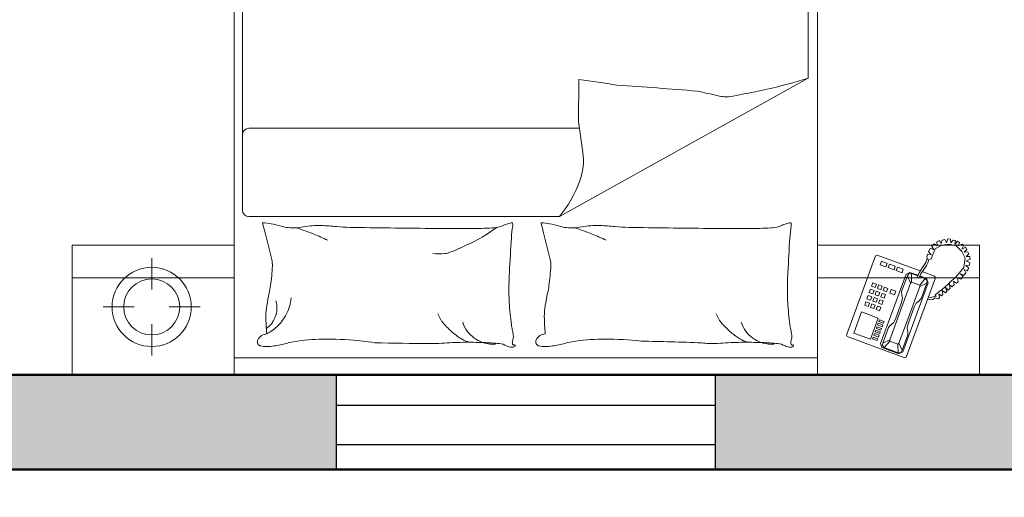
# Model space of a CAD drawing. Units: inches. Extents: x -7 to 1228, y -146 to 1091.
# Tile 17 of 88: x 420 to 513, y 57 to 103. Entities that reach past the tile are written whole.
import ezdxf

# ---------------------------------------------------------------- set-up
doc = ezdxf.new("R2010")
doc.units = ezdxf.units.IN
for name, color, linetype, lineweight in [('A-ANNO-DIMS', 2, 'Continuous', 18), ('A-FURN', 8, 'Continuous', 18), ('A-GLAZ', 175, 'Continuous', 25), ('A-WALL', 7, 'Continuous', 50), ('A-WALL-PATT', 251, 'Continuous', 13)]:
    doc.layers.add(name, color=color, linetype=linetype, lineweight=lineweight)
doc.styles.add('DIM_FONT', font='SIMPLEX.shx', dxfattribs={"width": 0.8})
doc.styles.get("Standard").update_dxf_attribs({"font": 'arial.ttf'})
doc.dimstyles.new('ISO-25', dxfattribs={"dimtxt": 7, "dimasz": 4, "dimexe": 1.25, "dimexo": 0.625, "dimtad": 1, "dimdec": 1, "dimlunit": 3, "dimtxsty": 'Standard', "dimcen": 2.5, "dimadec": 0, "dimazin": 0, "dimtfac": 1, "dimtdec": 1, "dimtmove": 1, "dimatfit": 3, "dimfxl": 1, "dimarcsym": 0})

# ---------------------------------------------------------------- blocks, each defined once
blk = doc.blocks.new('A$C4F634EDD')
for p, q in [((0, 2.6295), (0, 2.2295)), ((0.5, 2.6295), (0, 2.6295)), ((0.5, 2.6295), (2.3, 2.6295)), ((0.5, 0.5295), (0.5, 2.6295)), ((0.5, 2.2295), (0.5, 2.6295)), ((2.3, 2.6295), (2.3, 0.5295)), ((2.3, 2.6295), (2.8, 2.6295)), ((2.3, 2.2295), (2.3, 2.6295)), ((2.8, 2.6295), (2.8, 2.2295)), ((0.2457, 2.5697), (0.2457, 2.4733)), ((0.5, 2.5771), (2.3, 2.5771)), ((2.392, 2.5115), (2.5692, 2.5765)), ((2.4985, 2.5445), (2.5516, 2.564)), ((2.5062, 2.5454), (2.5487, 2.561)), ((2.5483, 2.5347), (2.5487, 2.561)), ((2.5487, 2.561), (2.5571, 2.56)), ((2.5615, 2.5536), (2.5514, 2.5318)), ((2.5516, 2.564), (2.5637, 2.5584)), ((2.5571, 2.56), (2.5615, 2.5536)), ((2.5615, 2.5536), (2.5791, 2.5058)), ((2.5637, 2.5584), (2.6418, 2.3458)), ((2.5692, 2.5765), (2.574, 2.5743)), ((2.574, 2.5743), (2.6638, 2.3298)), ((2.4842, 2.5232), (2.47, 2.518)), ((2.4862, 2.5179), (2.4842, 2.5232)), ((2.4946, 2.5331), (2.4985, 2.5445)), ((2.5734, 2.3187), (2.4946, 2.5331)), ((2.5062, 2.5454), (2.5004, 2.5392)), ((2.5004, 2.5392), (2.5013, 2.5315)), ((2.5013, 2.5315), (2.5188, 2.4836)), ((2.5013, 2.5315), (2.5231, 2.5214)), ((2.5235, 2.5256), (2.5062, 2.5454)), ((2.5231, 2.5214), (2.5235, 2.5256)), ((2.5483, 2.5347), (2.5235, 2.5256)), ((2.5514, 2.5318), (2.5483, 2.5347)), ((2.5807, 2.4521), (2.5514, 2.5318)), ((2.3898, 2.5066), (2.392, 2.5115)), ((2.4795, 2.2621), (2.3898, 2.5066)), ((2.412, 2.5007), (2.4634, 2.5196)), ((2.4361, 2.4352), (2.412, 2.5007)), ((2.4634, 2.5196), (2.4875, 2.454)), ((2.47, 2.518), (2.472, 2.5127)), ((2.472, 2.5127), (2.4862, 2.5179)), ((2.4881, 2.5126), (2.4739, 2.5074)), ((2.4739, 2.5074), (2.4759, 2.502)), ((2.4759, 2.502), (2.4901, 2.5073)), ((2.492, 2.5019), (2.4778, 2.4967)), ((2.4778, 2.4967), (2.4798, 2.4914)), ((2.4798, 2.4914), (2.494, 2.4966)), ((2.4901, 2.5073), (2.4881, 2.5126)), ((2.494, 2.4966), (2.492, 2.5019)), ((2.5523, 2.4417), (2.5231, 2.5214)), ((2.5788, 2.4956), (2.5767, 2.4848)), ((2.5791, 2.5058), (2.5788, 2.4956)), ((2.4959, 2.4913), (2.4817, 2.4861)), ((2.4817, 2.4861), (2.4837, 2.4808)), ((2.4837, 2.4808), (2.4979, 2.486)), ((2.4998, 2.4807), (2.4856, 2.4755)), ((2.4856, 2.4755), (2.4876, 2.4702)), ((2.4876, 2.4702), (2.5018, 2.4754)), ((2.5037, 2.47), (2.4895, 2.4648)), ((2.4895, 2.4648), (2.4915, 2.4595)), ((2.4915, 2.4595), (2.5057, 2.4647)), ((2.4979, 2.486), (2.4959, 2.4913)), ((2.5018, 2.4754), (2.4998, 2.4807)), ((2.5057, 2.4647), (2.5037, 2.47)), ((2.5188, 2.4836), (2.5256, 2.4761)), ((2.5256, 2.4761), (2.5342, 2.4692)), ((2.5342, 2.4692), (2.5405, 2.4574)), ((2.5767, 2.4848), (2.5795, 2.4717)), ((2.5795, 2.4717), (2.586, 2.454)), ((2.4875, 2.454), (2.4361, 2.4352)), ((2.4811, 2.4276), (2.4917, 2.4315)), ((2.4917, 2.4315), (2.4956, 2.4208)), ((2.5405, 2.4574), (2.547, 2.4397)), ((2.5594, 2.4061), (2.547, 2.4397)), ((2.5523, 2.4417), (2.5875, 2.346)), ((2.5807, 2.4521), (2.6158, 2.3564)), ((2.5984, 2.4204), (2.586, 2.454)), ((0.0957, 2.4197), (0.192, 2.4197)), ((0.2994, 2.4197), (0.3957, 2.4197)), ((2.4457, 2.4146), (2.4563, 2.4185)), ((2.4496, 2.4039), (2.4457, 2.4146)), ((2.4602, 2.4078), (2.4496, 2.4039)), ((2.4563, 2.4185), (2.4602, 2.4078)), ((2.4634, 2.4211), (2.474, 2.425)), ((2.4673, 2.4104), (2.4634, 2.4211)), ((2.4779, 2.4143), (2.4673, 2.4104)), ((2.4706, 2.4016), (2.4812, 2.4055)), ((2.4745, 2.3909), (2.4706, 2.4016)), ((2.474, 2.425), (2.4779, 2.4143)), ((2.485, 2.4169), (2.4811, 2.4276)), ((2.4812, 2.4055), (2.4851, 2.3949)), ((2.4956, 2.4208), (2.485, 2.4169)), ((2.4883, 2.4081), (2.4989, 2.412)), ((2.4922, 2.3975), (2.4883, 2.4081)), ((2.5028, 2.4014), (2.4922, 2.3975)), ((2.4989, 2.412), (2.5028, 2.4014)), ((2.5622, 2.393), (2.5594, 2.4061)), ((2.6047, 2.4086), (2.5984, 2.4204)), ((2.6133, 2.4017), (2.6047, 2.4086)), ((2.6201, 2.3941), (2.6133, 2.4017)), ((2.4528, 2.3951), (2.4635, 2.399)), ((2.4567, 2.3844), (2.4528, 2.3951)), ((2.4674, 2.3883), (2.4567, 2.3844)), ((2.46, 2.3756), (2.4706, 2.3795)), ((2.4639, 2.365), (2.46, 2.3756)), ((2.4635, 2.399), (2.4674, 2.3883)), ((2.4706, 2.3795), (2.4745, 2.3689)), ((2.4851, 2.3949), (2.4745, 2.3909)), ((2.4777, 2.3821), (2.4883, 2.386)), ((2.4816, 2.3715), (2.4777, 2.3821)), ((2.4922, 2.3754), (2.4816, 2.3715)), ((2.4883, 2.386), (2.4922, 2.3754)), ((2.4954, 2.3886), (2.5061, 2.3925)), ((2.4993, 2.378), (2.4954, 2.3886)), ((2.51, 2.3819), (2.4993, 2.378)), ((2.5026, 2.3691), (2.5132, 2.373)), ((2.5061, 2.3925), (2.51, 2.3819)), ((2.5132, 2.373), (2.5171, 2.3624)), ((2.5238, 2.3769), (2.538, 2.3821)), ((2.5277, 2.3663), (2.5238, 2.3769)), ((2.5419, 2.3715), (2.5277, 2.3663)), ((2.538, 2.3821), (2.5419, 2.3715)), ((2.5598, 2.372), (2.5601, 2.3822)), ((2.5774, 2.3242), (2.5598, 2.372)), ((2.5601, 2.3822), (2.5622, 2.393)), ((2.6376, 2.3463), (2.6201, 2.3941)), ((2.6499, 2.3979), (2.6397, 2.3953)), ((2.6417, 2.39), (2.6488, 2.391)), ((2.6488, 2.391), (2.6538, 2.3895)), ((2.6551, 2.397), (2.6499, 2.3979)), ((2.6538, 2.3895), (2.6596, 2.388)), ((2.6627, 2.392), (2.6551, 2.397)), ((2.6596, 2.388), (2.6626, 2.3867)), ((2.6626, 2.3867), (2.6662, 2.388)), ((2.6692, 2.394), (2.6627, 2.392)), ((2.6662, 2.388), (2.6632, 2.3828)), ((2.6632, 2.3828), (2.6736, 2.3744)), ((2.6736, 2.3944), (2.6692, 2.394)), ((2.6765, 2.391), (2.6736, 2.3944)), ((2.6736, 2.3744), (2.6922, 2.3593)), ((2.6742, 2.3795), (2.6765, 2.391)), ((2.6824, 2.3858), (2.6742, 2.3795)), ((2.6873, 2.3815), (2.6824, 2.3858)), ((2.6853, 2.369), (2.6873, 2.3815)), ((2.6946, 2.376), (2.6853, 2.369)), ((2.6995, 2.3713), (2.6946, 2.376)), ((2.695, 2.3603), (2.6995, 2.3713)), ((0.2457, 2.366), (0.2457, 2.2697)), ((2.4745, 2.3689), (2.4639, 2.365)), ((2.4672, 2.3561), (2.4778, 2.36)), ((2.4711, 2.3455), (2.4672, 2.3561)), ((2.4817, 2.3494), (2.4711, 2.3455)), ((2.4778, 2.36), (2.4817, 2.3494)), ((2.4849, 2.3626), (2.4955, 2.3665)), ((2.4888, 2.352), (2.4849, 2.3626)), ((2.4994, 2.3559), (2.4888, 2.352)), ((2.4955, 2.3665), (2.4994, 2.3559)), ((2.5065, 2.3585), (2.5026, 2.3691)), ((2.5171, 2.3624), (2.5065, 2.3585)), ((2.5774, 2.3242), (2.5875, 2.346)), ((2.5875, 2.346), (2.5905, 2.3431)), ((2.5905, 2.3431), (2.5901, 2.3168)), ((2.6154, 2.3522), (2.5905, 2.3431)), ((2.6158, 2.3564), (2.6154, 2.3522)), ((2.6154, 2.3522), (2.6327, 2.3324)), ((2.6376, 2.3463), (2.6158, 2.3564)), ((2.6418, 2.3458), (2.6369, 2.332)), ((2.6385, 2.3386), (2.6376, 2.3463)), ((2.6922, 2.3593), (2.7051, 2.3473)), ((2.7031, 2.3682), (2.695, 2.3603)), ((2.7096, 2.3616), (2.7031, 2.3682)), ((2.7051, 2.3473), (2.7079, 2.3475)), ((2.7062, 2.351), (2.7096, 2.3616)), ((2.7147, 2.3578), (2.7062, 2.351)), ((2.7079, 2.3475), (2.7079, 2.3443)), ((2.7079, 2.3443), (2.727, 2.3277)), ((2.7214, 2.3517), (2.7147, 2.3578)), ((2.7196, 2.34), (2.7214, 2.3517)), ((2.7286, 2.3466), (2.7196, 2.34)), ((2.7346, 2.3423), (2.7286, 2.3466)), ((2.732, 2.3295), (2.7346, 2.3423)), ((0, 2.3301), (0.5, 2.3301)), ((2.8, 2.3301), (2.3, 2.3301)), ((2.561, 2.3141), (2.5433, 2.3076)), ((2.5649, 2.3035), (2.561, 2.3141)), ((2.5855, 2.3131), (2.5734, 2.3187)), ((2.5818, 2.3178), (2.5774, 2.3242)), ((2.5901, 2.3168), (2.5818, 2.3178)), ((2.6104, 2.3222), (2.5855, 2.3131)), ((2.5901, 2.3168), (2.6097, 2.324)), ((2.613, 2.3312), (2.6077, 2.3293)), ((2.6077, 2.3293), (2.6135, 2.3141)), ((2.6192, 2.3174), (2.613, 2.3312)), ((2.6135, 2.3141), (2.6244, 2.2977)), ((2.6153, 2.3261), (2.6327, 2.3324)), ((2.6369, 2.332), (2.6161, 2.3243)), ((2.626, 2.3069), (2.6192, 2.3174)), ((2.6616, 2.3249), (2.6234, 2.3109)), ((2.6327, 2.3324), (2.6385, 2.3386)), ((2.6638, 2.3298), (2.6616, 2.3249)), ((2.727, 2.3277), (2.7512, 2.2983)), ((2.7423, 2.3345), (2.732, 2.3295)), ((2.7406, 2.3172), (2.7495, 2.325)), ((2.7519, 2.3218), (2.7406, 2.3172)), ((2.7495, 2.325), (2.7423, 2.3345)), ((2.7575, 2.3144), (2.7519, 2.3218)), ((2.7526, 2.3045), (2.7575, 2.3144)), ((2.6172, 2.3086), (2.4844, 2.2599)), ((2.5114, 2.2959), (2.4936, 2.2894)), ((2.4936, 2.2894), (2.4976, 2.2788)), ((2.4976, 2.2788), (2.5153, 2.2853)), ((2.5153, 2.2853), (2.5114, 2.2959)), ((2.5362, 2.305), (2.5185, 2.2985)), ((2.5185, 2.2985), (2.5224, 2.2879)), ((2.5224, 2.2879), (2.5401, 2.2944)), ((2.5401, 2.2944), (2.5362, 2.305)), ((2.5433, 2.3076), (2.5472, 2.297)), ((2.5472, 2.297), (2.5649, 2.3035)), ((2.6244, 2.2977), (2.6349, 2.2825)), ((2.6365, 2.2916), (2.626, 2.3069)), ((2.6349, 2.2825), (2.638, 2.273)), ((2.6407, 2.2834), (2.6365, 2.2916)), ((2.6438, 2.2739), (2.6407, 2.2834)), ((2.7512, 2.2983), (2.756, 2.2695)), ((2.7622, 2.308), (2.7526, 2.3045)), ((2.7574, 2.2924), (2.7673, 2.2997)), ((2.7687, 2.2905), (2.7574, 2.2924)), ((2.7587, 2.279), (2.7699, 2.2828)), ((2.7708, 2.2725), (2.7587, 2.279)), ((2.7673, 2.2997), (2.7622, 2.308)), ((2.7699, 2.2828), (2.7687, 2.2905)), ((0.5953, 2.1912), (0.616, 2.2738)), ((1.4546, 2.1912), (1.4752, 2.2738)), ((2.4844, 2.2599), (2.4795, 2.2621)), ((2.6399, 2.2712), (2.6374, 2.2659)), ((2.6374, 2.2659), (2.6398, 2.257)), ((2.638, 2.273), (2.6399, 2.2712)), ((2.6398, 2.257), (2.6509, 2.259)), ((2.6509, 2.259), (2.6431, 2.2492)), ((2.6431, 2.2492), (2.6473, 2.2398)), ((2.6519, 2.2716), (2.6438, 2.2739)), ((2.6535, 2.2628), (2.6519, 2.2716)), ((2.6636, 2.2409), (2.6535, 2.2628)), ((2.7459, 2.2483), (2.7284, 2.2317)), ((2.756, 2.2695), (2.7459, 2.2483)), ((2.7529, 2.2505), (2.7645, 2.2498)), ((2.7607, 2.2424), (2.7529, 2.2505)), ((2.759, 2.2637), (2.7706, 2.2643)), ((2.7676, 2.2559), (2.759, 2.2637)), ((2.7645, 2.2498), (2.7676, 2.2559)), ((2.7706, 2.2643), (2.7708, 2.2725)), ((0, 2.2295), (0.5, 2.2295)), ((2.8, 2.2295), (2.3, 2.2295)), ((2.6473, 2.2398), (2.6592, 2.2429)), ((2.6592, 2.2429), (2.6521, 2.2314)), ((2.6521, 2.2314), (2.6598, 2.2248)), ((2.6598, 2.2248), (2.6697, 2.2309)), ((2.6836, 2.2287), (2.6636, 2.2409)), ((2.6697, 2.2309), (2.6684, 2.219)), ((2.6684, 2.219), (2.6761, 2.2145)), ((2.6761, 2.2145), (2.6821, 2.2237)), ((2.6821, 2.2237), (2.6843, 2.2135)), ((2.7063, 2.2256), (2.6836, 2.2287)), ((2.6927, 2.2117), (2.6986, 2.222)), ((2.6986, 2.222), (2.7019, 2.2098)), ((2.7284, 2.2317), (2.7063, 2.2256)), ((2.7102, 2.2104), (2.7113, 2.2218)), ((2.7113, 2.2218), (2.7192, 2.2137)), ((2.7255, 2.2152), (2.7242, 2.2265)), ((2.7242, 2.2265), (2.7324, 2.2165)), ((2.7324, 2.2165), (2.7386, 2.2208)), ((2.7386, 2.2208), (2.7354, 2.2306)), ((2.7354, 2.2306), (2.7462, 2.2264)), ((2.7509, 2.2314), (2.7459, 2.2418)), ((2.7459, 2.2418), (2.7568, 2.2352)), ((2.7462, 2.2264), (2.7509, 2.2314)), ((2.7568, 2.2352), (2.7607, 2.2424)), ((0.5878, 2.1612), (0.5953, 2.1912)), ((1.4471, 2.1612), (1.4546, 2.1912)), ((2.6843, 2.2135), (2.6927, 2.2117)), ((2.7019, 2.2098), (2.7102, 2.2104)), ((2.7192, 2.2137), (2.7255, 2.2152)), ((1.5035, 2.141), (0.5458, 2.141)), ((1.5035, 2.141), (2.2716, 1.7136)), ((0.5258, 2.121), (0.5258, 0.5617)), ((1.576, 1.9433), (1.5624, 1.8479)), ((0.5458, 1.8684), (1.5653, 1.8684)), ((1.5624, 1.8479), (1.5641, 1.7178)), ((2.2716, 0.5617), (2.2716, 1.7136))]:
    blk.add_line(p, q)
for radius in [0.1222, 0.0865]:
    blk.add_circle((0.2457, 2.4197), radius)
for centre, radius, start, end in [((0.5848, 2.5274), 0.0131, 101.2724, 206.5805), ((0.5999, 2.4516), 0.0904, 90, 101.2724), ((0.5999, 2.3808), 0.1611, 81.5628, 90), ((0.5788, 2.2388), 0.3048, 74.256, 81.5628), ((0.7272, 2.7653), 0.2422, 254.256, 262.4531), ((0.7851, 3.2019), 0.6827, 262.4531, 270), ((0.7851, 3.5682), 1.049, 270, 276.0867), ((0.8402, 3.0514), 0.5293, 276.0867, 280.1899), ((1.1602, -8.1346), 10.6675, 90.30153, 91.21582), ((1.1169, 2.2433), 0.2897, 85.1982, 92.5386), ((1.2142, 3.4021), 0.8732, 265.1982, 269.4243), ((1.3082, 2.3102), 0.234, 110.8603, 117.2396), ((1.2204, 4.0232), 1.4943, 269.4243, 271.9079), ((1.2995, 2.4357), 0.0992, 105.9352, 126.0864), ((1.2429, 3.3501), 0.8208, 271.9079, 275.2592), ((1.2995, 2.4357), 0.0992, 85.7841, 105.9352), ((1.3132, 2.5864), 0.0539, 275.2592, 300.6513), ((1.3554, 2.5152), 0.0289, 85.6975, 120.6513), ((1.3556, 2.519), 0.0251, 68.2117, 85.6975), ((1.3739, 2.5288), 0.0156, 158.0096, 201.421), ((1.3634, 2.533), 0.00428, 78.1069, 158.0096), ((1.3288, 2.5111), 0.0328, 351.8665, 21.421), ((1.3647, 2.5395), 0.00232, 258.1069, 19.564), ((1.3637, 2.5391), 0.00342, 19.564, 68.2117), ((1.444, 2.5274), 0.0131, 101.2724, 206.5805), ((1.4591, 2.4516), 0.0904, 90, 101.2724), ((1.4591, 2.3808), 0.1611, 81.5628, 90), ((1.438, 2.2388), 0.3048, 74.256, 81.5628), ((1.5865, 2.7653), 0.2422, 254.256, 262.4531), ((1.6443, 3.2019), 0.6827, 262.4531, 270), ((1.6443, 3.5682), 1.049, 270, 276.0867), ((1.4785, 15.4878), 12.9656, 271.22425, 272.05324), ((1.97, 2.3805), 0.1524, 92.5386, 100.1899), ((1.9761, 2.2433), 0.2897, 85.1982, 92.5386), ((2.0734, 3.4021), 0.8732, 265.1982, 269.4243), ((2.1674, 2.3102), 0.234, 110.8603, 117.2396), ((2.0797, 4.0232), 1.4943, 269.4243, 271.9079), ((2.1588, 2.4357), 0.0992, 105.9352, 126.0864), ((2.1021, 3.3501), 0.8208, 271.9079, 275.2592), ((2.1588, 2.4357), 0.0992, 85.7841, 105.9352), ((2.1724, 2.5864), 0.0539, 275.2592, 300.6513), ((2.2146, 2.5152), 0.0289, 85.6975, 120.6513), ((2.2149, 2.519), 0.0251, 68.2117, 85.6975), ((2.2331, 2.5288), 0.0156, 158.0096, 201.421), ((2.2226, 2.533), 0.00428, 78.1069, 158.0096), ((2.1881, 2.5111), 0.0328, 351.8665, 21.421), ((2.224, 2.5395), 0.00232, 258.1069, 19.564), ((2.2229, 2.5391), 0.00342, 19.564, 68.2117), ((0.6036, 2.5368), 0.0342, 206.5805, 265.5998), ((1.0898, 2.4496), 0.4918, 173.7676, 180), ((0.5368, 2.3783), 0.1399, 45.0976, 62.7964), ((1.4317, 2.2032), 0.3916, 128.3886, 133.8115), ((1.2362, 2.45), 0.0768, 117.2396, 128.3886), ((1.2995, 2.4357), 0.0992, 143.8234, 161.5603), ((1.2995, 2.4357), 0.0992, 126.0864, 143.8234), ((1.1177, 2.5413), 0.246, 347.8905, 351.8665), ((1.4628, 2.5368), 0.0342, 206.5805, 265.5998), ((1.949, 2.4496), 0.4918, 173.7676, 180), ((2.291, 2.2032), 0.3916, 128.3886, 133.8115), ((2.0954, 2.45), 0.0768, 117.2396, 128.3886), ((2.1588, 2.4357), 0.0992, 143.8234, 161.5603), ((2.1588, 2.4357), 0.0992, 126.0864, 143.8234), ((1.977, 2.5413), 0.246, 347.8905, 351.8665), ((0.5462, 2.4142), 0.0899, 41.4429, 53.7359), ((0.5741, 2.4389), 0.0526, 25.3551, 41.4429), ((0.4851, 2.3967), 0.1511, 21.8149, 25.3551), ((0.5368, 2.3783), 0.1399, 27.3988, 45.0976), ((1.1799, 2.4341), 0.0493, 140.9651, 151.6832), ((1.3165, 2.3233), 0.2252, 133.8115, 140.9651), ((2.2605, 2.3525), 0.9131, 172.3191, 176.6313), ((1.5522, 2.448), 0.1983, 167.8905, 172.3191), ((2.0391, 2.4341), 0.0493, 140.9651, 151.6832), ((2.1757, 2.3233), 0.2252, 133.8115, 140.9651), ((3.1198, 2.3525), 0.9131, 172.3191, 176.6313), ((2.4114, 2.448), 0.1983, 167.8905, 172.3191), ((0.8019, 2.4496), 0.204, 180, 189.6844), ((0.4345, 2.3765), 0.2056, 18.7799, 21.8149), ((0.576, 2.4246), 0.0562, 0, 18.7799), ((0.5368, 2.3783), 0.1399, 16.515, 27.3988), ((1.3127, 2.3625), 0.2002, 151.6832, 156.9972), ((1.6611, 2.4496), 0.204, 180, 189.6844), ((2.1719, 2.3625), 0.2002, 151.6832, 156.9972), ((1.4703, 2.5637), 0.882, 189.6844, 192.1984), ((0.5406, 2.4246), 0.0915, 345.3149, 0), ((0.5368, 2.3783), 0.1399, 5.6311, 16.515), ((2.0266, 2.3663), 0.6787, 176.6313, 181.6331), ((2.3295, 2.5637), 0.882, 189.6844, 192.1984), ((2.8858, 2.3663), 0.6787, 176.6313, 181.6331), ((0.2982, 2.3103), 0.3171, 8.0051, 12.1984), ((1.1575, 2.3103), 0.3171, 8.0051, 12.1984), ((-0.0401, 2.2627), 0.6588, 2.6649, 8.0051), ((2.7128, 2.3859), 1.3652, 181.6331, 183.055), ((0.8191, 2.2627), 0.6588, 2.6649, 8.0051), ((3.5721, 2.3859), 1.3652, 181.6331, 183.055), ((14.9657, 3.0398), 13.6356, 183.05496, 183.50486), ((15.8249, 3.0398), 13.6356, 183.05496, 183.50486), ((0.5503, 2.2902), 0.0677, 345.9548, 2.6649), ((1.4096, 2.2902), 0.0677, 345.9548, 2.6649), ((1.1303, 1.9835), 0.2721, 85.9172, 93.5552), ((1.1455, 2.197), 0.058, 69.3257, 85.9172), ((0.9871, 1.7772), 0.5066, 65.6735, 69.3257), ((0.6058, 0.9338), 1.4323, 63.5015, 65.6735), ((0.473, 2.8815), 0.7387, 289.428, 291.6577), ((0.473, 2.8815), 0.7387, 291.6577, 293.4844), ((0.473, 2.8815), 0.7387, 293.4844, 295.3111), ((1.1054, 1.9358), 0.3126, 57.865, 63.5015), ((0.8841, 1.5835), 0.7286, 54.1737, 57.865), ((1.6762, 2.2258), 0.3212, 183.5049, 189.9984), ((1.3322, 2.8815), 0.7387, 289.428, 291.6577), ((1.3322, 2.8815), 0.7387, 291.6577, 293.4844), ((1.3322, 2.8815), 0.7387, 293.4844, 295.3111), ((2.5355, 2.2258), 0.3212, 183.5049, 189.9984), ((0.5887, 2.1609), 0.000917, 165.9551, 274.0829), ((0.5695, 2.4301), 0.2708, 274.0829, 279.4841), ((0.5763, 2.3896), 0.2297, 279.4841, 287.3864), ((0.6807, 2.0561), 0.1197, 96.4341, 107.3864), ((0.6836, 2.0301), 0.1459, 78.4414, 96.4341), ((0.473, 2.8815), 0.7387, 287.1982, 289.428), ((0.759, 2.3985), 0.2301, 258.4414, 272.7491), ((0.7026, 3.5718), 1.4048, 272.7491, 274.6176), ((0.9136, 0.9591), 1.2165, 92.6096, 94.6176), ((1.2501, -19.8405), 22.0183, 90.37908, 91.01965), ((1.2012, -3.5404), 5.7185, 89.7135, 90.9704), ((1.224, 1.0141), 1.164, 86.426, 89.7135), ((1.2875, 2.0302), 0.1459, 77.131, 86.426), ((1.3099, 2.1283), 0.0453, 62.7159, 77.131), ((1.3658, 2.2367), 0.0767, 242.7159, 253.7788), ((1.3688, 2.247), 0.0875, 253.7788, 262.8796), ((1.3581, 2.1615), 0.00132, 262.8796, 343.3022), ((1.3409, 2.1667), 0.0193, 343.3022, 9.9984), ((1.448, 2.1609), 0.000917, 165.9551, 274.0829), ((1.4288, 2.4301), 0.2708, 274.0829, 279.4841), ((1.4355, 2.3896), 0.2297, 279.4841, 287.3864), ((1.5399, 2.0561), 0.1197, 96.4341, 107.3864), ((1.5429, 2.0301), 0.1459, 78.4414, 96.4341), ((1.3322, 2.8815), 0.7387, 287.1982, 289.428), ((1.6182, 2.3985), 0.2301, 258.4414, 272.7491), ((1.5619, 3.5718), 1.4048, 272.7491, 274.6176), ((1.7729, 0.9591), 1.2165, 92.6096, 94.6176), ((2.1093, -19.8405), 22.0183, 90.37908, 91.01965), ((2.0605, -3.5404), 5.7185, 89.7135, 90.9704), ((2.0833, 1.0141), 1.164, 86.426, 89.7135), ((2.1467, 2.0302), 0.1459, 77.131, 86.426), ((2.1691, 2.1283), 0.0453, 62.7159, 77.131), ((2.2251, 2.2367), 0.0767, 242.7159, 253.7788), ((2.2281, 2.247), 0.0875, 253.7788, 262.8796), ((2.2174, 2.1615), 0.00132, 262.8796, 343.3022), ((2.2001, 2.1667), 0.0193, 343.3022, 9.9984), ((0.5458, 2.121), 0.02, 90, 180), ((1.2147, 1.9017), 0.3751, 20.1488, 39.6445), ((1.3977, 1.9688), 0.1801, 351.8644, 20.1488), ((0.5458, 1.8884), 0.02, 180, 270), ((1.4194, 4.2174), 2.5158, 281.6741, 283.1904), ((2.0378, 1.5789), 0.1942, 97.7304, 103.1904), ((2.0195, 1.7137), 0.0581, 79.2724, 97.7304), ((1.2737, -2.2227), 4.0646, 77.0745, 79.2724), ((1.0582, 5.4638), 3.7801, 277.692, 279.495), ((0.6102, 18.0525), 16.3521, 273.75703, 274.62393), ((2.0359, 1.0981), 0.6574, 74.0648, 77.0745), ((1.7125, -0.0344), 1.8351, 72.2636, 74.0648)]:
    blk.add_arc(centre, radius, start, end)
at = {"style": 'DIM_FONT', "width": 0.8, "flags": 9}
for tag, p in [('YSIZE', (0.5, 2.6295)), ('XSIZE', (0.5, 2.6295)), ('XSIZE', (2.2985, 2.6295)), ('YSIZE', (2.2985, 2.6295))]:
    blk.add_attdef(tag, p, '', height=0.0005, dxfattribs=at)
blk = doc.blocks.new('WIN-36')
for p, q in [((0, 36), (0, 0)), ((9, 36), (0, 36)), ((2.343, 36), (2.343, 0)), ((6.137, 0), (6.137, 36)), ((9, 0), (9, 36)), ((0, 0), (9, 0)), ((2.343, 0), (6.137, 0))]:
    blk.add_line(p, q)
blk = doc.blocks.new('*D38')
at = {"layer": 'A-ANNO-DIMS', "color": 0, "lineweight": -2, "transparency": 16777216}
for p, q in [((324.905, 55.362), (324.905, 47.508)), ((373.098, 55.362), (373.098, 47.508)), ((328.905, 48.758), (369.098, 48.758)), ((349.002, 48.758), (352.917, 35.705)), ((352.917, 35.705), (500.857, 35.705))]:
    blk.add_line(p, q, dxfattribs=at)
at = {"layer": 'A-ANNO-DIMS', "color": 0, "transparency": 16777216}
for points in [[(328.905, 49.424), (328.905, 48.091), (324.905, 48.758)], [(369.098, 49.424), (369.098, 48.091), (373.098, 48.758)]]:
    blk.add_solid(points, dxfattribs=at)
at = {"layer": 'Defpoints', "color": 0, "transparency": 16777216}
for p in [(324.905, 55.987), (373.098, 55.987), (373.098, 48.758)]:
    blk.add_point(p, dxfattribs=at)
at = {"layer": 'A-ANNO-DIMS', "color": 0, "transparency": 16777216, "insert": (426.887, 39.952), "char_height": 7, "attachment_point": 5}
blk.add_mtext('BALCONY CHAIR SET 4\'-0" TYP.', dxfattribs=at)

msp = doc.modelspace()

# ---------------------------------------------------------------- hatches: boundary and pattern name
at = {"layer": 'A-WALL-PATT'}
h = msp.add_hatch(color=256, dxfattribs=at)
h.dxf.hatch_style = 1
h.paths.add_polyline_path([(69, 568), (60, 568), (60, 493), (63.289, 493), (69, 493)])
h.paths.add_polyline_path([(69, 662.405), (60, 662.405), (60, 586), (69, 586)], flags=17)
h.paths.add_polyline_path([(69, 723), (184, 723), (184, 734), (179, 734), (179, 728), (69, 728), (69, 741.623), (60, 741.623), (60, 698.405), (69, 698.405)], flags=17)
h.paths.add_polyline_path([(69, 782), (231, 782), (231, 728), (231, 723), (231, 586), (236, 586), (236, 787), (69, 787), (69, 800.126), (60, 800.126), (60, 765.623), (69, 765.623)])
h.paths.add_polyline_path([(184, 842), (189, 842), (189, 848), (173, 848), (173, 842), (179, 842), (179, 787), (184, 787)])
h.paths.add_polyline_path([(118.22, 69), (69, 69), (69, 60), (118.22, 60)])
h.paths.add_polyline_path([(227, 69), (154.22, 69), (154.22, 60), (227, 60)])
h.paths.add_polyline_path([(236, 60), (232.711, 60), (227, 60), (227, 36), (236, 36)])
h.paths.add_polyline_path([(389, 60), (380, 60), (380, 36), (389, 36)])
h.paths.add_polyline_path([(384, 181), (380, 181), (380, 115), (380, 78), (384, 78)])
h.paths.add_polyline_path([(380, 115), (334.547, 115), (334.547, 109), (380, 109)])
h.paths.add_polyline_path([(274.547, 115), (236, 115), (236, 201), (232.711, 201), (231, 201), (231, 78), (236, 78), (236, 109), (274.547, 109)])
h.paths.add_polyline_path([(69, 123), (60, 123), (60, 78), (69, 78)])
h.paths.add_polyline_path([(69, 201), (60, 201), (60, 159), (69, 159)])
h.paths.add_polyline_path([(143, 219), (69, 219), (69, 213), (143, 213)], flags=17)
h.paths.add_polyline_path([(189, 219), (184, 219), (184, 274), (231, 274), (231, 219), (236, 219), (236, 279), (184, 279), (184, 297), (179, 297), (179, 279), (69, 279), (69, 290.912), (60, 290.912), (60, 262.179), (69, 262.179), (69, 274), (179, 274), (179, 219), (173, 219), (173, 213), (189, 213)])
h.paths.add_polyline_path([(69, 238.179), (60, 238.179), (60, 219), (69, 219)], flags=17)
h.paths.add_polyline_path([(69, 333), (60, 333), (60, 314.912), (69, 314.912), (69, 316.965)])
h.paths.add_polyline_path([(190, 338), (184, 338), (69, 338), (69, 333), (179, 333), (179, 327), (184, 327), (184, 333.021), (190, 333.046)])
h.paths.add_polyline_path([(69, 386.806), (60, 386.806), (60, 351), (69, 351)])
h.paths.add_polyline_path([(69, 475), (60, 475), (60, 422.806), (69, 422.806)])
h.paths.add_polyline_path([(236, 475), (231, 475), (231, 351.238), (236, 351.238)])
h.paths.add_polyline_path([(384, 475), (380, 475), (380, 362), (384, 362)])
h.paths.add_polyline_path([(547, 307), (439, 307), (439, 356), (445, 356), (445, 362), (433, 362), (433, 307), (380, 307), (380, 244), (380, 241), (384, 241), (384, 301), (433, 301), (433, 277), (439, 277), (439, 301), (547, 301)])
h.paths.add_polyline_path([(547, 241), (439, 241), (439, 247), (433, 247), (433, 235), (547, 235)])
h.paths.add_polyline_path([(450, 69), (440.286, 69), (424.889, 69), (389, 69), (389, 60), (450, 60)])
h.paths.add_polyline_path([(547, 69), (486, 69), (486, 60), (547, 60)])
h.paths.add_polyline_path([(556, 148.268), (547, 148.268), (547, 78), (556, 78)])
h.paths.add_polyline_path([(556, 223), (547, 223), (547, 195), (547, 184.268), (556, 184.268)])
h.paths.add_polyline_path([(556, 311.192), (547, 311.192), (547, 273.075), (556, 273.075)])
h.paths.add_polyline_path([(556, 344), (552.711, 344), (547, 344), (547, 335.192), (556, 335.192)])
h.paths.add_polyline_path([(556, 249.075), (547, 249.075), (547, 241), (556, 241)])
h.paths.add_polyline_path([(547, 362), (475, 362), (475, 356), (547, 356)], flags=0)
h.paths.add_polyline_path([(556, 399.621), (547, 399.621), (547, 362), (556, 362)])
h.paths.add_polyline_path([(556, 475), (547, 475), (547, 435.621), (556, 435.621)])
h.paths.add_polyline_path([(547, 493), (389, 493), (389, 487), (547, 487)])
h.paths.add_polyline_path([(380, 493), (278, 493), (278, 487), (380, 487)])
h.paths.add_polyline_path([(227, 493), (69, 493), (69, 487), (227, 487)])
h.paths.add_polyline_path([(643, 122.445), (634, 122.445), (634, 78), (643, 78)])
h.paths.add_polyline_path([(702.5, 69), (692.786, 69), (677.389, 69), (643, 69), (643, 60), (702.5, 60)])
h.paths.add_polyline_path([(798, 69), (738.5, 69), (738.5, 60), (798, 60)])
h.paths.add_polyline_path([(807, 60), (803.711, 60), (798, 60), (798, 36), (807, 36)])
h.paths.add_polyline_path([(807, 109), (846.751, 109), (846.751, 115), (807, 115), (807, 159), (802, 159), (802, 78), (807, 78)])
h.paths.add_polyline_path([(807, 201), (802, 201), (802, 195), (807, 195)])
h.paths.add_polyline_path([(643, 201), (634, 201), (634, 158.445), (643, 158.445)])
h.paths.add_polyline_path([(756, 225), (751, 225), (751, 219), (643, 219), (643, 213), (756, 213)])
h.paths.add_polyline_path([(643, 240.848), (634, 240.848), (634, 219), (643, 219)])
h.paths.add_polyline_path([(643, 274), (643, 288.629), (634, 288.629), (634, 264.848), (643, 264.848)])
h.paths.add_polyline_path([(802, 279), (756, 279), (756, 297), (751, 297), (751, 279), (643, 279), (643, 274), (751, 274), (751, 255), (756, 255), (756, 274), (802, 274)])
h.paths.add_polyline_path([(807, 333), (803.711, 333), (802, 333), (802, 279), (802, 274), (802, 219), (807, 219)])
h.paths.add_polyline_path([(956, 182), (951, 182), (951, 115), (906.751, 115), (906.751, 109), (951, 109), (951, 78), (956, 78)])
h.paths.add_polyline_path([(960, 60), (951, 60), (951, 36), (960, 36)])
h.paths.add_polyline_path([(1021, 69), (1005.781, 69), (960, 69), (960, 60), (1021, 60)])
h.paths.add_polyline_path([(956, 224), (951, 224), (951, 218), (956, 218)])
h.paths.add_polyline_path([(956, 302), (1004, 302), (1004, 278), (1010, 278), (1010, 302), (1118, 302), (1118, 290.809), (1127, 290.809), (1127, 326.968), (1118, 326.968), (1118, 320.966), (1118, 307), (1010, 307), (1010, 356), (1016, 356), (1016, 362), (1004, 362), (1004, 307), (951, 307), (951, 244), (951, 242), (954.289, 242), (956, 242)])
h.paths.add_polyline_path([(643, 333), (634, 333), (634, 312.629), (643, 312.629), (643, 316.965)])
h.paths.add_polyline_path([(756, 338), (643, 338), (643, 333), (751, 333), (751, 327), (756, 327)])
h.paths.add_polyline_path([(643, 388), (634, 388), (634, 351), (643, 351)])
h.paths.add_polyline_path([(807, 357), (802, 357), (802, 351), (807, 351)])
h.paths.add_polyline_path([(807, 475), (802, 475), (802, 393), (807, 393)])
h.paths.add_polyline_path([(643, 475), (634, 475), (634, 424), (643, 424)])
h.paths.add_polyline_path([(798, 493), (643, 493), (643, 487), (798, 487)])
h.paths.add_polyline_path([(634, 493), (556, 493), (556, 487), (634, 487)])
h.paths.add_polyline_path([(813, 493), (807, 493), (807, 487), (813, 487)])
h.paths.add_polyline_path([(951, 493), (849, 493), (849, 487), (951, 487)])
h.paths.add_polyline_path([(956, 484), (951, 484), (951, 374), (956, 374)])
h.paths.add_polyline_path([(1109, 493), (969, 493), (969, 487), (1109, 487)])
h.paths.add_polyline_path([(1127, 484), (1118, 484), (1118, 450.641), (1127, 450.641)])
h.paths.add_polyline_path([(1127, 414.641), (1118, 414.641), (1118, 365), (1127, 365)])
h.paths.add_polyline_path([(1109, 362), (1046, 362), (1046, 356), (1109, 356)], flags=17)
h.paths.add_polyline_path([(1127, 356), (1123.454, 356), (1118, 356), (1118, 350.968), (1127, 350.968)], flags=0)
h.paths.add_polyline_path([(1127, 266.809), (1118, 266.809), (1118, 262.361), (1118, 242), (1127, 242)], flags=17)
h.paths.add_polyline_path([(1118, 242), (1010, 242), (1010, 248), (1004, 248), (1004, 237), (1118, 237)])
h.paths.add_polyline_path([(1127, 224), (1118, 224), (1118, 170), (1127, 170)])
h.paths.add_polyline_path([(1127, 134), (1118, 134), (1118, 78), (1127, 78)])
h.paths.add_polyline_path([(1118, 69), (1057, 69), (1057, 60), (1118, 60)])
h.paths.add_polyline_path([(227, 571.546), (227, 574), (69, 574), (69, 568), (227, 568)])
h.paths.add_polyline_path([(380, 571.546), (380, 574), (278, 574), (278, 568), (380, 568)])
h.paths.add_polyline_path([(242, 574), (236, 574), (236, 568), (242, 568)])
h.paths.add_polyline_path([(547, 571.546), (547, 574), (389, 574), (389, 568), (547, 568)])
h.paths.add_polyline_path([(384, 733), (380, 733), (380, 586), (384, 586)])
h.paths.add_polyline_path([(556, 646), (634, 646), (634, 655), (547, 655), (547, 586), (556, 586)])
h.paths.add_polyline_path([(634, 574), (556, 574), (556, 568), (634, 568)])
h.paths.add_polyline_path([(643, 655), (634, 655), (634, 586), (643, 586)])
h.paths.add_polyline_path([(798, 574), (643, 574), (643, 568), (798, 568)])
h.paths.add_polyline_path([(643, 663.854), (634, 663.854), (634, 655), (643, 655)])
h.paths.add_polyline_path([(556, 676.967), (547, 676.967), (547, 655), (556, 655)])
h.paths.add_polyline_path([(556, 733), (547, 733), (547, 712.967), (556, 712.967)])
h.paths.add_polyline_path([(643, 710), (634, 710), (634, 699.854), (643, 699.854)])
h.paths.add_polyline_path([(807, 668), (802, 668), (802, 586), (807, 586)])
h.paths.add_polyline_path([(951, 574), (849, 574), (849, 568), (951, 568)])
h.paths.add_polyline_path([(956, 691), (951, 691), (951, 577), (956, 577)])
h.paths.add_polyline_path([(1109, 574), (969, 574), (969, 568), (1109, 568)])
h.paths.add_polyline_path([(1127, 643.403), (1118, 643.403), (1118, 577), (1127, 577)])
h.paths.add_polyline_path([(1127, 568), (1123.454, 568), (1118, 568), (1118, 493), (1127, 493)])
h.paths.add_polyline_path([(1127, 733), (1118, 733), (1118, 679.403), (1127, 679.403)])
h.paths.add_polyline_path([(1127, 777.348), (1118, 777.348), (1118, 770.035), (1118, 751), (1127, 751)], flags=17)
h.paths.add_polyline_path([(1118, 751), (1010, 751), (1010, 757), (1004, 757), (1004, 745), (1118, 745)])
h.paths.add_polyline_path([(956, 811), (1004, 811), (1004, 787), (1010, 787), (1010, 811), (1017.874, 811), (1017.874, 811.627, -0.414214), (1018.247, 812), (1031.978, 812, -0.414214), (1032.351, 811.627), (1032.351, 811), (1118, 811), (1118, 801.348), (1127, 801.348), (1127, 834.685), (1118, 834.685), (1118, 830.238), (1118, 817), (1010, 817), (1010, 866), (1016, 866), (1016, 872), (1004, 872), (1004, 817), (956, 817), (956, 866), (951, 866), (951, 751), (954.289, 751), (956, 751)])
h.paths.add_polyline_path([(1118, 872), (1046, 872), (1046, 866), (1118, 866)], flags=17)
h.paths.add_polyline_path([(1127, 924.711), (1118, 924.711), (1118, 884), (1127, 884)])
h.paths.add_polyline_path([(1127, 866), (1123.711, 866), (1118, 866), (1118, 858.685), (1127, 858.685)], flags=17)
h.paths.add_polyline_path([(956, 983), (951, 983), (951, 952), (807, 952), (807, 983), (802, 983), (802, 902), (807, 902), (807, 946), (951, 946), (951, 884), (956, 884)])
h.paths.add_polyline_path([(807, 842), (802, 842), (802, 787), (756, 787), (756, 806), (751, 806), (751, 787), (643, 787), (643, 782), (751, 782), (751, 764), (756, 764), (756, 782), (802, 782), (802, 728), (807, 728)])
h.paths.add_polyline_path([(756, 848), (643, 848), (643, 842), (751, 842), (751, 836), (756, 836)])
h.paths.add_polyline_path([(756, 734), (751, 734), (751, 728), (643, 728), (643, 723), (756, 723)])
h.paths.add_polyline_path([(643, 749.791), (634, 749.791), (634, 728), (637.289, 728), (643, 728)])
h.paths.add_polyline_path([(643, 805.405), (634, 805.405), (634, 773.791), (643, 773.791)])
h.paths.add_polyline_path([(643, 896.663), (634, 896.663), (634, 860), (637.289, 860), (643, 860)])
h.paths.add_polyline_path([(643, 842), (634, 842), (634, 829.405), (643, 829.405)])
h.paths.add_polyline_path([(643, 983), (634, 983), (634, 932.663), (643, 932.663)])
h.paths.add_polyline_path([(1127, 983), (1118, 983), (1118, 960.711), (1127, 960.711)])
h.paths.add_polyline_path([(1118, 1001), (1077.525, 1001), (1077.525, 992), (1118, 992)])
h.paths.add_polyline_path([(1041.525, 1001), (960, 1001), (960, 992), (1041.525, 992)])
h.paths.add_polyline_path([(960, 1025), (951, 1025), (951, 1001), (954.289, 1001), (960, 1001)])
h.paths.add_polyline_path([(807, 1025), (798, 1025), (798, 1001), (807, 1001)])
h.paths.add_polyline_path([(798, 1001), (738.5, 1001), (738.5, 992), (798, 992)])
h.paths.add_polyline_path([(702.5, 1001), (643, 1001), (643, 992), (702.5, 992)])
h.paths.add_polyline_path([(547, 1001), (499.113, 1001), (499.113, 992), (547, 992)])
h.paths.add_polyline_path([(463.113, 1001), (389, 1001), (389, 992), (463.113, 992)])
h.paths.add_polyline_path([(389, 1025), (380, 1025), (380, 1022), (380, 1001), (383.289, 1001), (389, 1001)])
h.paths.add_polyline_path([(236, 1025), (227, 1025), (227, 1001), (236, 1001)])
h.paths.add_polyline_path([(236, 983), (231, 983), (231, 860), (236, 860)])
h.paths.add_polyline_path([(274.547, 952), (236, 952), (236, 946), (274.547, 946)])
h.paths.add_polyline_path([(380, 952), (334.547, 952), (334.547, 946), (380, 946)])
h.paths.add_polyline_path([(384, 983), (380, 983), (380, 884), (383.289, 884), (384, 884)])
h.paths.add_polyline_path([(227, 1001), (155.012, 1001), (155.012, 992), (162.875, 992), (227, 992)])
h.paths.add_polyline_path([(119.012, 1001), (69, 1001), (69, 992), (119.012, 992)])
h.paths.add_polyline_path([(69, 983), (60, 983), (60, 922.987), (69, 922.987)])
h.paths.add_polyline_path([(69, 886.987), (60, 886.987), (60, 860), (63.289, 860), (69, 860)])
h.paths.add_polyline_path([(143, 848), (69, 848), (69, 842), (143, 842)])

# ---------------------------------------------------------------- linework, layer by layer
at = {"layer": 'A-WALL'}
for p, q in [((556, 69), (380, 69)), ((556, 60), (380, 60)), ((380, 60), (807, 60))]:
    msp.add_line(p, q, dxfattribs=at)

# ---------------------------------------------------------------- block references
at = {"layer": 'A-FURN', "xscale": -30.79356024027943, "yscale": 30.79356024027943, "zscale": 30.79356024027943, "rotation": 180}
msp.add_blockref('A$C4F634EDD', (424.889, 149.972), dxfattribs=at)
at = {"layer": 'A-GLAZ', "extrusion": (0, 0, -1), "zscale": -1, "rotation": 89.99999999999994}
msp.add_blockref('WIN-36', (-450, 60), dxfattribs=at)

# ---------------------------------------------------------------- dimensions: what is measured, and where the dimension line sits
at = {"layer": 'A-ANNO-DIMS'}
dim = msp.add_linear_dim(base=(373.098, 48.758), p1=(324.905, 55.987), p2=(373.098, 55.987), text='BALCONY CHAIR SET <> TYP.', dimstyle='ISO-25', override={"dimdec": 1, "dimlfac": 1, "dimrnd": 0, "dimzin": 1, "dimdsep": 46, "dimlunit": 4, "dimfrac": 2}, dxfattribs=at)
dim.commit()
dim.dimension.update_dxf_attribs({"geometry": '*D38', "text_midpoint": (353.542, 39.952)})

doc.saveas('drawing.dxf')
